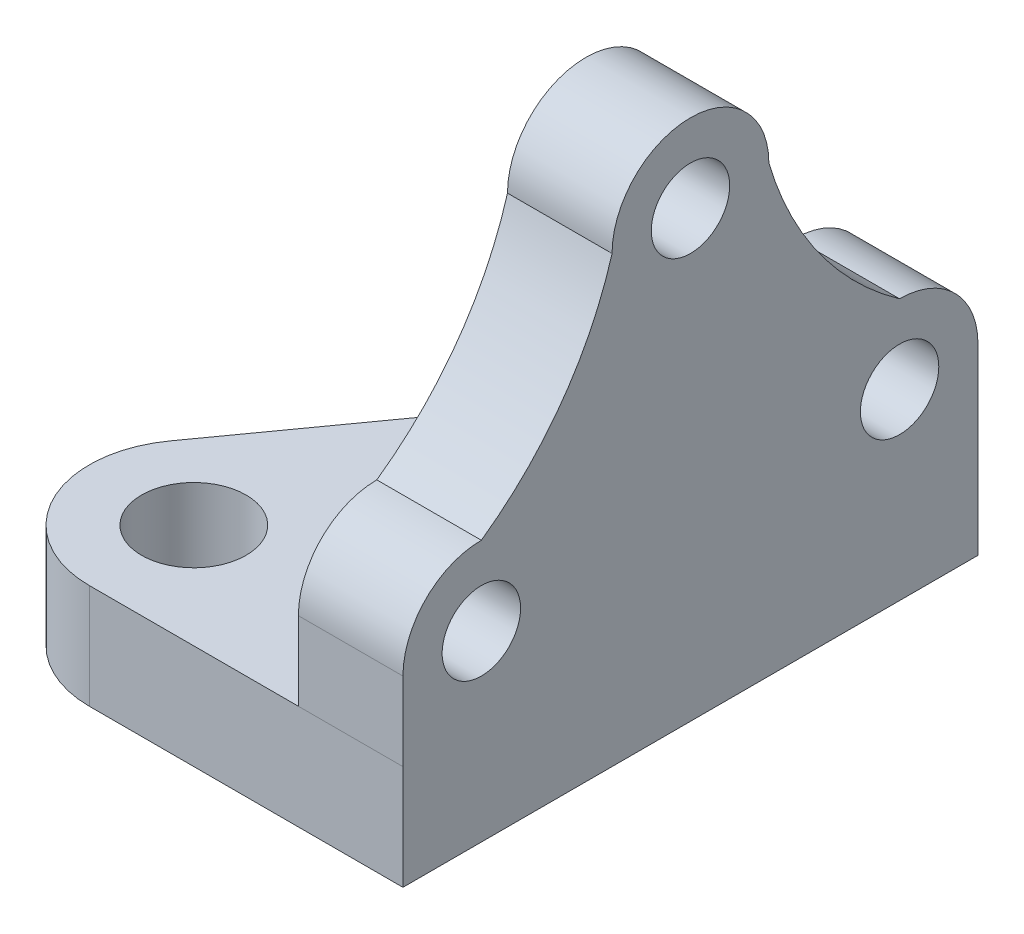
ISO-10303-21;
HEADER;
FILE_DESCRIPTION(('STEP AP214'),'2;1');
FILE_NAME('part.step','',(''),(''),'','','');
FILE_SCHEMA(('AUTOMOTIVE_DESIGN { 1 0 10303 214 1 1 1 1 }'));
ENDSEC;
DATA;
#1=APPLICATION_CONTEXT('core data for automotive mechanical design processes');
#2=APPLICATION_PROTOCOL_DEFINITION('international standard','automotive_design',2000,#1);
#3=PRODUCT_CONTEXT('',#1,'mechanical');
#4=PRODUCT('Part','Part','',(#3));
#5=PRODUCT_RELATED_PRODUCT_CATEGORY('part','',(#4));
#6=PRODUCT_DEFINITION_FORMATION('','',#4);
#7=PRODUCT_DEFINITION_CONTEXT('part definition',#1,'design');
#8=PRODUCT_DEFINITION('design','',#6,#7);
#9=PRODUCT_DEFINITION_SHAPE('','',#8);
#10=(LENGTH_UNIT() NAMED_UNIT(*) SI_UNIT(.MILLI.,.METRE.));
#11=(NAMED_UNIT(*) PLANE_ANGLE_UNIT() SI_UNIT($,.RADIAN.));
#12=(NAMED_UNIT(*) SI_UNIT($,.STERADIAN.) SOLID_ANGLE_UNIT());
#13=UNCERTAINTY_MEASURE_WITH_UNIT(LENGTH_MEASURE(1.E-05),#10,'distance_accuracy_value','');
#14=(GEOMETRIC_REPRESENTATION_CONTEXT(3) GLOBAL_UNCERTAINTY_ASSIGNED_CONTEXT((#13)) GLOBAL_UNIT_ASSIGNED_CONTEXT((#10,
#11,#12)) REPRESENTATION_CONTEXT('',''));
#15=CARTESIAN_POINT('',(0.,0.,0.));
#16=DIRECTION('',(0.,0.,1.));
#17=DIRECTION('',(1.,0.,0.));
#18=AXIS2_PLACEMENT_3D('',#15,#16,#17);
#19=CARTESIAN_POINT('',(20.,68.1526978623619,-77.4137770073067));
#20=DIRECTION('',(1.,0.,0.));
#21=DIRECTION('',(0.,0.,-1.));
#22=AXIS2_PLACEMENT_3D('',#19,#20,#21);
#23=PLANE('',#22);
#24=CARTESIAN_POINT('',(20.,0.,-40.));
#25=DIRECTION('',(1.,0.,0.));
#26=DIRECTION('',(0.,0.,-1.));
#27=AXIS2_PLACEMENT_3D('',#24,#25,#26);
#28=CIRCLE('',#27,7.5);
#29=CARTESIAN_POINT('',(20.,0.,-47.5));
#30=VERTEX_POINT('',#29);
#31=EDGE_CURVE('E154',#30,#30,#28,.T.);
#32=ORIENTED_EDGE('',*,*,#31,.F.);
#33=EDGE_LOOP('',(#32));
#34=FACE_BOUND('',#33,.T.);
#35=CARTESIAN_POINT('',(20.,68.1526978623619,-77.4137770073067));
#36=DIRECTION('',(-1.,0.,0.));
#37=DIRECTION('',(0.,0.,-1.));
#38=AXIS2_PLACEMENT_3D('',#35,#36,#37);
#39=CIRCLE('',#38,65.);
#40=CARTESIAN_POINT('',(20.,15.,-40.));
#41=VERTEX_POINT('',#40);
#42=CARTESIAN_POINT('',(20.,50.,-15.));
#43=VERTEX_POINT('',#42);
#44=EDGE_CURVE('E170',#41,#43,#39,.T.);
#45=ORIENTED_EDGE('',*,*,#44,.T.);
#46=CARTESIAN_POINT('',(20.,50.,0.));
#47=DIRECTION('',(1.,0.,0.));
#48=DIRECTION('',(0.,0.,-1.));
#49=AXIS2_PLACEMENT_3D('',#46,#47,#48);
#50=CIRCLE('',#49,15.);
#51=CARTESIAN_POINT('',(20.,50.,15.));
#52=VERTEX_POINT('',#51);
#53=EDGE_CURVE('E100',#43,#52,#50,.T.);
#54=ORIENTED_EDGE('',*,*,#53,.T.);
#55=CARTESIAN_POINT('',(20.,68.1526978623619,77.4137770073067));
#56=DIRECTION('',(-1.,0.,0.));
#57=DIRECTION('',(0.,0.,1.));
#58=AXIS2_PLACEMENT_3D('',#55,#56,#57);
#59=CIRCLE('',#58,65.);
#60=CARTESIAN_POINT('',(20.,15.,40.));
#61=VERTEX_POINT('',#60);
#62=EDGE_CURVE('E168',#52,#61,#59,.T.);
#63=ORIENTED_EDGE('',*,*,#62,.T.);
#64=CARTESIAN_POINT('',(20.,0.,40.));
#65=DIRECTION('',(1.,0.,0.));
#66=DIRECTION('',(0.,0.,-1.));
#67=AXIS2_PLACEMENT_3D('',#64,#65,#66);
#68=CIRCLE('',#67,15.);
#69=CARTESIAN_POINT('',(20.,0.,55.));
#70=VERTEX_POINT('',#69);
#71=EDGE_CURVE('E116',#61,#70,#68,.T.);
#72=ORIENTED_EDGE('',*,*,#71,.T.);
#73=DIRECTION('',(0.,-0.999999995009303,9.9906924504711E-05));
#74=VECTOR('',#73,1.);
#75=CARTESIAN_POINT('',(20.,-15.,55.001498603875));
#76=LINE('',#75,#74);
#77=CARTESIAN_POINT('',(20.,-15.,55.001498603875));
#78=VERTEX_POINT('',#77);
#79=EDGE_CURVE('E112',#70,#78,#76,.T.);
#80=ORIENTED_EDGE('',*,*,#79,.T.);
#81=DIRECTION('',(0.,1.,0.));
#82=VECTOR('',#81,1.);
#83=CARTESIAN_POINT('',(20.,-35.,55.001498603875));
#84=LINE('',#83,#82);
#85=CARTESIAN_POINT('',(20.,-35.,55.001498603875));
#86=VERTEX_POINT('',#85);
#87=EDGE_CURVE('E119',#86,#78,#84,.T.);
#88=ORIENTED_EDGE('',*,*,#87,.F.);
#89=DIRECTION('',(0.,0.,1.));
#90=VECTOR('',#89,1.);
#91=CARTESIAN_POINT('',(20.,-35.,-55.));
#92=LINE('',#91,#90);
#93=CARTESIAN_POINT('',(20.,-35.,-55.));
#94=VERTEX_POINT('',#93);
#95=EDGE_CURVE('E415',#94,#86,#92,.T.);
#96=ORIENTED_EDGE('',*,*,#95,.F.);
#97=DIRECTION('',(0.,1.,0.));
#98=VECTOR('',#97,1.);
#99=CARTESIAN_POINT('',(20.,0.,-55.));
#100=LINE('',#99,#98);
#101=CARTESIAN_POINT('',(20.,0.,-55.));
#102=VERTEX_POINT('',#101);
#103=EDGE_CURVE('E122',#94,#102,#100,.T.);
#104=ORIENTED_EDGE('',*,*,#103,.T.);
#105=CARTESIAN_POINT('',(20.,0.,-40.));
#106=DIRECTION('',(1.,0.,0.));
#107=DIRECTION('',(0.,0.,-1.));
#108=AXIS2_PLACEMENT_3D('',#105,#106,#107);
#109=CIRCLE('',#108,15.);
#110=EDGE_CURVE('E57',#102,#41,#109,.T.);
#111=ORIENTED_EDGE('',*,*,#110,.T.);
#112=EDGE_LOOP('',(#45,#54,#63,#72,#80,#88,#96,#104,#111));
#113=FACE_BOUND('',#112,.T.);
#114=CARTESIAN_POINT('',(20.,50.,0.));
#115=DIRECTION('',(1.,0.,0.));
#116=DIRECTION('',(0.,0.,-1.));
#117=AXIS2_PLACEMENT_3D('',#114,#115,#116);
#118=CIRCLE('',#117,7.5);
#119=CARTESIAN_POINT('',(20.,50.,-7.5));
#120=VERTEX_POINT('',#119);
#121=EDGE_CURVE('E161',#120,#120,#118,.T.);
#122=ORIENTED_EDGE('',*,*,#121,.F.);
#123=EDGE_LOOP('',(#122));
#124=FACE_BOUND('',#123,.T.);
#125=CARTESIAN_POINT('',(20.,0.,40.));
#126=DIRECTION('',(1.,0.,0.));
#127=DIRECTION('',(0.,0.,-1.));
#128=AXIS2_PLACEMENT_3D('',#125,#126,#127);
#129=CIRCLE('',#128,7.5);
#130=CARTESIAN_POINT('',(20.,0.,32.5));
#131=VERTEX_POINT('',#130);
#132=EDGE_CURVE('E144',#131,#131,#129,.T.);
#133=ORIENTED_EDGE('',*,*,#132,.F.);
#134=EDGE_LOOP('',(#133));
#135=FACE_BOUND('',#134,.T.);
#136=ADVANCED_FACE('F39',(#34,#113,#124,#135),#23,.T.);
#137=CARTESIAN_POINT('',(0.,68.1526978623619,-77.4137770073067));
#138=DIRECTION('',(1.,0.,0.));
#139=DIRECTION('',(0.,0.,-1.));
#140=AXIS2_PLACEMENT_3D('',#137,#138,#139);
#141=PLANE('',#140);
#142=CARTESIAN_POINT('',(0.,68.1526978623619,-77.4137770073067));
#143=DIRECTION('',(-1.,0.,0.));
#144=DIRECTION('',(0.,0.,-1.));
#145=AXIS2_PLACEMENT_3D('',#142,#143,#144);
#146=CIRCLE('',#145,65.);
#147=CARTESIAN_POINT('',(0.,15.,-40.));
#148=VERTEX_POINT('',#147);
#149=CARTESIAN_POINT('',(0.,50.,-15.));
#150=VERTEX_POINT('',#149);
#151=EDGE_CURVE('E163',#148,#150,#146,.T.);
#152=ORIENTED_EDGE('',*,*,#151,.F.);
#153=CARTESIAN_POINT('',(0.,0.,-40.));
#154=DIRECTION('',(1.,0.,0.));
#155=DIRECTION('',(0.,0.,-1.));
#156=AXIS2_PLACEMENT_3D('',#153,#154,#155);
#157=CIRCLE('',#156,15.);
#158=CARTESIAN_POINT('',(0.,0.,-55.));
#159=VERTEX_POINT('',#158);
#160=EDGE_CURVE('E90',#159,#148,#157,.T.);
#161=ORIENTED_EDGE('',*,*,#160,.F.);
#162=DIRECTION('',(0.,1.,0.));
#163=VECTOR('',#162,1.);
#164=CARTESIAN_POINT('',(0.,0.,-55.));
#165=LINE('',#164,#163);
#166=CARTESIAN_POINT('',(0.,-15.,-55.));
#167=VERTEX_POINT('',#166);
#168=EDGE_CURVE('E83',#167,#159,#165,.T.);
#169=ORIENTED_EDGE('',*,*,#168,.F.);
#170=DIRECTION('',(0.,0.,-1.));
#171=VECTOR('',#170,1.);
#172=CARTESIAN_POINT('',(0.,-15.,-55.));
#173=LINE('',#172,#171);
#174=CARTESIAN_POINT('',(0.,-15.,55.001498603875));
#175=VERTEX_POINT('',#174);
#176=EDGE_CURVE('E183',#175,#167,#173,.T.);
#177=ORIENTED_EDGE('',*,*,#176,.F.);
#178=DIRECTION('',(0.,-0.999999995009303,9.9906924504711E-05));
#179=VECTOR('',#178,1.);
#180=CARTESIAN_POINT('',(0.,-15.,55.001498603875));
#181=LINE('',#180,#179);
#182=CARTESIAN_POINT('',(0.,0.,55.));
#183=VERTEX_POINT('',#182);
#184=EDGE_CURVE('E128',#183,#175,#181,.T.);
#185=ORIENTED_EDGE('',*,*,#184,.F.);
#186=CARTESIAN_POINT('',(0.,0.,40.));
#187=DIRECTION('',(1.,0.,0.));
#188=DIRECTION('',(0.,0.,-1.));
#189=AXIS2_PLACEMENT_3D('',#186,#187,#188);
#190=CIRCLE('',#189,15.);
#191=CARTESIAN_POINT('',(0.,15.,40.));
#192=VERTEX_POINT('',#191);
#193=EDGE_CURVE('E185',#192,#183,#190,.T.);
#194=ORIENTED_EDGE('',*,*,#193,.F.);
#195=CARTESIAN_POINT('',(0.,68.1526978623619,77.4137770073067));
#196=DIRECTION('',(-1.,0.,0.));
#197=DIRECTION('',(0.,0.,1.));
#198=AXIS2_PLACEMENT_3D('',#195,#196,#197);
#199=CIRCLE('',#198,65.);
#200=CARTESIAN_POINT('',(0.,50.,15.));
#201=VERTEX_POINT('',#200);
#202=EDGE_CURVE('E179',#201,#192,#199,.T.);
#203=ORIENTED_EDGE('',*,*,#202,.F.);
#204=CARTESIAN_POINT('',(0.,50.,0.));
#205=DIRECTION('',(1.,0.,0.));
#206=DIRECTION('',(0.,0.,-1.));
#207=AXIS2_PLACEMENT_3D('',#204,#205,#206);
#208=CIRCLE('',#207,15.);
#209=EDGE_CURVE('E178',#150,#201,#208,.T.);
#210=ORIENTED_EDGE('',*,*,#209,.F.);
#211=EDGE_LOOP('',(#152,#161,#169,#177,#185,#194,#203,#210));
#212=FACE_BOUND('',#211,.T.);
#213=CARTESIAN_POINT('',(0.,50.,0.));
#214=DIRECTION('',(1.,0.,0.));
#215=DIRECTION('',(0.,0.,-1.));
#216=AXIS2_PLACEMENT_3D('',#213,#214,#215);
#217=CIRCLE('',#216,7.5);
#218=CARTESIAN_POINT('',(0.,50.,-7.5));
#219=VERTEX_POINT('',#218);
#220=EDGE_CURVE('E158',#219,#219,#217,.T.);
#221=ORIENTED_EDGE('',*,*,#220,.T.);
#222=EDGE_LOOP('',(#221));
#223=FACE_BOUND('',#222,.T.);
#224=CARTESIAN_POINT('',(0.,0.,-40.));
#225=DIRECTION('',(1.,0.,0.));
#226=DIRECTION('',(0.,0.,-1.));
#227=AXIS2_PLACEMENT_3D('',#224,#225,#226);
#228=CIRCLE('',#227,7.5);
#229=CARTESIAN_POINT('',(0.,0.,-47.5));
#230=VERTEX_POINT('',#229);
#231=EDGE_CURVE('E153',#230,#230,#228,.T.);
#232=ORIENTED_EDGE('',*,*,#231,.T.);
#233=EDGE_LOOP('',(#232));
#234=FACE_BOUND('',#233,.T.);
#235=CARTESIAN_POINT('',(0.,0.,40.));
#236=DIRECTION('',(1.,0.,0.));
#237=DIRECTION('',(0.,0.,-1.));
#238=AXIS2_PLACEMENT_3D('',#235,#236,#237);
#239=CIRCLE('',#238,7.5);
#240=CARTESIAN_POINT('',(0.,0.,32.5));
#241=VERTEX_POINT('',#240);
#242=EDGE_CURVE('E143',#241,#241,#239,.T.);
#243=ORIENTED_EDGE('',*,*,#242,.T.);
#244=EDGE_LOOP('',(#243));
#245=FACE_BOUND('',#244,.T.);
#246=ADVANCED_FACE('F204',(#212,#223,#234,#245),#141,.F.);
#247=CARTESIAN_POINT('',(20.,68.1526978623619,-77.4137770073067));
#248=DIRECTION('',(-1.,0.,0.));
#249=DIRECTION('',(0.,0.,1.));
#250=AXIS2_PLACEMENT_3D('',#247,#248,#249);
#251=CYLINDRICAL_SURFACE('',#250,65.);
#252=ORIENTED_EDGE('',*,*,#151,.T.);
#253=DIRECTION('',(-1.,0.,0.));
#254=VECTOR('',#253,1.);
#255=CARTESIAN_POINT('',(20.,50.,-15.));
#256=LINE('',#255,#254);
#257=EDGE_CURVE('E11',#43,#150,#256,.T.);
#258=ORIENTED_EDGE('',*,*,#257,.F.);
#259=ORIENTED_EDGE('',*,*,#44,.F.);
#260=DIRECTION('',(-1.,0.,0.));
#261=VECTOR('',#260,1.);
#262=CARTESIAN_POINT('',(20.,15.,-40.));
#263=LINE('',#262,#261);
#264=EDGE_CURVE('E171',#41,#148,#263,.T.);
#265=ORIENTED_EDGE('',*,*,#264,.T.);
#266=EDGE_LOOP('',(#252,#258,#259,#265));
#267=FACE_BOUND('',#266,.T.);
#268=ADVANCED_FACE('F41',(#267),#251,.F.);
#269=CARTESIAN_POINT('',(20.,50.,0.));
#270=DIRECTION('',(-1.,0.,0.));
#271=DIRECTION('',(0.,0.,1.));
#272=AXIS2_PLACEMENT_3D('',#269,#270,#271);
#273=CYLINDRICAL_SURFACE('',#272,15.);
#274=ORIENTED_EDGE('',*,*,#209,.T.);
#275=DIRECTION('',(-1.,0.,0.));
#276=VECTOR('',#275,1.);
#277=CARTESIAN_POINT('',(20.,50.,15.));
#278=LINE('',#277,#276);
#279=EDGE_CURVE('E48',#52,#201,#278,.T.);
#280=ORIENTED_EDGE('',*,*,#279,.F.);
#281=ORIENTED_EDGE('',*,*,#53,.F.);
#282=ORIENTED_EDGE('',*,*,#257,.T.);
#283=EDGE_LOOP('',(#274,#280,#281,#282));
#284=FACE_BOUND('',#283,.T.);
#285=ADVANCED_FACE('F220',(#284),#273,.T.);
#286=CARTESIAN_POINT('',(20.,68.1526978623619,77.4137770073067));
#287=DIRECTION('',(-1.,0.,0.));
#288=DIRECTION('',(0.,0.,1.));
#289=AXIS2_PLACEMENT_3D('',#286,#287,#288);
#290=CYLINDRICAL_SURFACE('',#289,65.);
#291=ORIENTED_EDGE('',*,*,#202,.T.);
#292=DIRECTION('',(-1.,0.,0.));
#293=VECTOR('',#292,1.);
#294=CARTESIAN_POINT('',(20.,15.,40.));
#295=LINE('',#294,#293);
#296=EDGE_CURVE('E193',#61,#192,#295,.T.);
#297=ORIENTED_EDGE('',*,*,#296,.F.);
#298=ORIENTED_EDGE('',*,*,#62,.F.);
#299=ORIENTED_EDGE('',*,*,#279,.T.);
#300=EDGE_LOOP('',(#291,#297,#298,#299));
#301=FACE_BOUND('',#300,.T.);
#302=ADVANCED_FACE('F200',(#301),#290,.F.);
#303=CARTESIAN_POINT('',(20.,0.,40.));
#304=DIRECTION('',(-1.,0.,0.));
#305=DIRECTION('',(0.,0.,1.));
#306=AXIS2_PLACEMENT_3D('',#303,#304,#305);
#307=CYLINDRICAL_SURFACE('',#306,15.);
#308=ORIENTED_EDGE('',*,*,#193,.T.);
#309=DIRECTION('',(-1.,0.,0.));
#310=VECTOR('',#309,1.);
#311=CARTESIAN_POINT('',(20.,0.,55.));
#312=LINE('',#311,#310);
#313=EDGE_CURVE('E135',#70,#183,#312,.T.);
#314=ORIENTED_EDGE('',*,*,#313,.F.);
#315=ORIENTED_EDGE('',*,*,#71,.F.);
#316=ORIENTED_EDGE('',*,*,#296,.T.);
#317=EDGE_LOOP('',(#308,#314,#315,#316));
#318=FACE_BOUND('',#317,.T.);
#319=ADVANCED_FACE('F210',(#318),#307,.T.);
#320=CARTESIAN_POINT('',(20.,-15.,55.001498603875));
#321=DIRECTION('',(0.,-9.9906924504711E-05,-0.999999995009303));
#322=DIRECTION('',(0.,0.999999995009303,-9.9906924504711E-05));
#323=AXIS2_PLACEMENT_3D('',#320,#321,#322);
#324=PLANE('',#323);
#325=ORIENTED_EDGE('',*,*,#184,.T.);
#326=DIRECTION('',(-1.,0.,0.));
#327=VECTOR('',#326,1.);
#328=CARTESIAN_POINT('',(20.,-15.,55.001498603875));
#329=LINE('',#328,#327);
#330=EDGE_CURVE('E130',#78,#175,#329,.T.);
#331=ORIENTED_EDGE('',*,*,#330,.F.);
#332=ORIENTED_EDGE('',*,*,#79,.F.);
#333=ORIENTED_EDGE('',*,*,#313,.T.);
#334=EDGE_LOOP('',(#325,#331,#332,#333));
#335=FACE_BOUND('',#334,.T.);
#336=ADVANCED_FACE('F126',(#335),#324,.F.);
#337=CARTESIAN_POINT('',(20.,0.,-55.));
#338=DIRECTION('',(0.,0.,1.));
#339=DIRECTION('',(1.,0.,0.));
#340=AXIS2_PLACEMENT_3D('',#337,#338,#339);
#341=PLANE('',#340);
#342=ORIENTED_EDGE('',*,*,#168,.T.);
#343=DIRECTION('',(-1.,0.,0.));
#344=VECTOR('',#343,1.);
#345=CARTESIAN_POINT('',(20.,0.,-55.));
#346=LINE('',#345,#344);
#347=EDGE_CURVE('E131',#102,#159,#346,.T.);
#348=ORIENTED_EDGE('',*,*,#347,.F.);
#349=ORIENTED_EDGE('',*,*,#103,.F.);
#350=DIRECTION('',(1.,0.,0.));
#351=VECTOR('',#350,1.);
#352=CARTESIAN_POINT('',(20.,-35.,-55.));
#353=LINE('',#352,#351);
#354=CARTESIAN_POINT('',(0.,-35.,-55.));
#355=VERTEX_POINT('',#354);
#356=EDGE_CURVE('E395',#355,#94,#353,.T.);
#357=ORIENTED_EDGE('',*,*,#356,.F.);
#358=DIRECTION('',(0.,1.,0.));
#359=VECTOR('',#358,1.);
#360=CARTESIAN_POINT('',(0.,-35.,-55.));
#361=LINE('',#360,#359);
#362=EDGE_CURVE('E393',#355,#167,#361,.T.);
#363=ORIENTED_EDGE('',*,*,#362,.T.);
#364=EDGE_LOOP('',(#342,#348,#349,#357,#363));
#365=FACE_BOUND('',#364,.T.);
#366=ADVANCED_FACE('F214',(#365),#341,.F.);
#367=CARTESIAN_POINT('',(20.,0.,-40.));
#368=DIRECTION('',(-1.,0.,0.));
#369=DIRECTION('',(0.,0.,1.));
#370=AXIS2_PLACEMENT_3D('',#367,#368,#369);
#371=CYLINDRICAL_SURFACE('',#370,15.);
#372=ORIENTED_EDGE('',*,*,#160,.T.);
#373=ORIENTED_EDGE('',*,*,#264,.F.);
#374=ORIENTED_EDGE('',*,*,#110,.F.);
#375=ORIENTED_EDGE('',*,*,#347,.T.);
#376=EDGE_LOOP('',(#372,#373,#374,#375));
#377=FACE_BOUND('',#376,.T.);
#378=ADVANCED_FACE('F235',(#377),#371,.T.);
#379=CARTESIAN_POINT('',(20.,50.,0.));
#380=DIRECTION('',(-1.,0.,0.));
#381=DIRECTION('',(0.,0.,1.));
#382=AXIS2_PLACEMENT_3D('',#379,#380,#381);
#383=CYLINDRICAL_SURFACE('',#382,7.5);
#384=ORIENTED_EDGE('',*,*,#121,.T.);
#385=EDGE_LOOP('',(#384));
#386=FACE_BOUND('',#385,.T.);
#387=ORIENTED_EDGE('',*,*,#220,.F.);
#388=EDGE_LOOP('',(#387));
#389=FACE_BOUND('',#388,.T.);
#390=ADVANCED_FACE('F230',(#386,#389),#383,.F.);
#391=CARTESIAN_POINT('',(20.,0.,-40.));
#392=DIRECTION('',(-1.,0.,0.));
#393=DIRECTION('',(0.,0.,1.));
#394=AXIS2_PLACEMENT_3D('',#391,#392,#393);
#395=CYLINDRICAL_SURFACE('',#394,7.5);
#396=ORIENTED_EDGE('',*,*,#31,.T.);
#397=EDGE_LOOP('',(#396));
#398=FACE_BOUND('',#397,.T.);
#399=ORIENTED_EDGE('',*,*,#231,.F.);
#400=EDGE_LOOP('',(#399));
#401=FACE_BOUND('',#400,.T.);
#402=ADVANCED_FACE('F306',(#398,#401),#395,.F.);
#403=CARTESIAN_POINT('',(20.,0.,40.));
#404=DIRECTION('',(-1.,0.,0.));
#405=DIRECTION('',(0.,0.,1.));
#406=AXIS2_PLACEMENT_3D('',#403,#404,#405);
#407=CYLINDRICAL_SURFACE('',#406,7.5);
#408=ORIENTED_EDGE('',*,*,#132,.T.);
#409=EDGE_LOOP('',(#408));
#410=FACE_BOUND('',#409,.T.);
#411=ORIENTED_EDGE('',*,*,#242,.F.);
#412=EDGE_LOOP('',(#411));
#413=FACE_BOUND('',#412,.T.);
#414=ADVANCED_FACE('F248',(#410,#413),#407,.F.);
#415=CARTESIAN_POINT('',(-40.,-15.,35.001498603875));
#416=DIRECTION('',(0.,-1.,0.));
#417=DIRECTION('',(0.,0.,-1.));
#418=AXIS2_PLACEMENT_3D('',#415,#416,#417);
#419=PLANE('',#418);
#420=CARTESIAN_POINT('',(-40.,-15.,35.001498603875));
#421=DIRECTION('',(0.,-1.,0.));
#422=DIRECTION('',(0.,0.,-1.));
#423=AXIS2_PLACEMENT_3D('',#420,#421,#422);
#424=CIRCLE('',#423,10.);
#425=CARTESIAN_POINT('',(-40.,-15.,25.001498603875));
#426=VERTEX_POINT('',#425);
#427=EDGE_CURVE('E418',#426,#426,#424,.T.);
#428=ORIENTED_EDGE('',*,*,#427,.T.);
#429=EDGE_LOOP('',(#428));
#430=FACE_BOUND('',#429,.T.);
#431=DIRECTION('',(-1.,0.,0.));
#432=VECTOR('',#431,1.);
#433=CARTESIAN_POINT('',(-40.,-15.,55.001498603875));
#434=LINE('',#433,#432);
#435=CARTESIAN_POINT('',(-40.,-15.,55.001498603875));
#436=VERTEX_POINT('',#435);
#437=EDGE_CURVE('E390',#175,#436,#434,.T.);
#438=ORIENTED_EDGE('',*,*,#437,.F.);
#439=ORIENTED_EDGE('',*,*,#176,.T.);
#440=DIRECTION('',(0.583235968180871,0.,-0.812302779399481));
#441=VECTOR('',#440,1.);
#442=CARTESIAN_POINT('',(0.,-15.,-55.));
#443=LINE('',#442,#441);
#444=CARTESIAN_POINT('',(-56.2460395562641,-15.,23.33675691208));
#445=VERTEX_POINT('',#444);
#446=EDGE_CURVE('E387',#445,#167,#443,.T.);
#447=ORIENTED_EDGE('',*,*,#446,.F.);
#448=CARTESIAN_POINT('',(-40.,-15.,35.001498603875));
#449=DIRECTION('',(0.,-1.,0.));
#450=DIRECTION('',(0.,0.,-1.));
#451=AXIS2_PLACEMENT_3D('',#448,#449,#450);
#452=CIRCLE('',#451,20.);
#453=EDGE_CURVE('E391',#436,#445,#452,.T.);
#454=ORIENTED_EDGE('',*,*,#453,.F.);
#455=EDGE_LOOP('',(#438,#439,#447,#454));
#456=FACE_BOUND('',#455,.T.);
#457=ADVANCED_FACE('F245',(#430,#456),#419,.F.);
#458=CARTESIAN_POINT('',(-40.,-35.,35.001498603875));
#459=DIRECTION('',(0.,-1.,0.));
#460=DIRECTION('',(0.,0.,-1.));
#461=AXIS2_PLACEMENT_3D('',#458,#459,#460);
#462=PLANE('',#461);
#463=ORIENTED_EDGE('',*,*,#356,.T.);
#464=ORIENTED_EDGE('',*,*,#95,.T.);
#465=DIRECTION('',(-1.,0.,0.));
#466=VECTOR('',#465,1.);
#467=CARTESIAN_POINT('',(20.,-35.,55.001498603875));
#468=LINE('',#467,#466);
#469=CARTESIAN_POINT('',(-40.,-35.,55.001498603875));
#470=VERTEX_POINT('',#469);
#471=EDGE_CURVE('E139',#86,#470,#468,.T.);
#472=ORIENTED_EDGE('',*,*,#471,.T.);
#473=CARTESIAN_POINT('',(-40.,-35.,35.001498603875));
#474=DIRECTION('',(0.,-1.,0.));
#475=DIRECTION('',(0.,0.,-1.));
#476=AXIS2_PLACEMENT_3D('',#473,#474,#475);
#477=CIRCLE('',#476,20.);
#478=CARTESIAN_POINT('',(-56.2460395562641,-35.,23.33675691208));
#479=VERTEX_POINT('',#478);
#480=EDGE_CURVE('E405',#470,#479,#477,.T.);
#481=ORIENTED_EDGE('',*,*,#480,.T.);
#482=DIRECTION('',(0.583235968180871,0.,-0.812302779399481));
#483=VECTOR('',#482,1.);
#484=CARTESIAN_POINT('',(0.,-35.,-55.));
#485=LINE('',#484,#483);
#486=EDGE_CURVE('E397',#479,#355,#485,.T.);
#487=ORIENTED_EDGE('',*,*,#486,.T.);
#488=EDGE_LOOP('',(#463,#464,#472,#481,#487));
#489=FACE_BOUND('',#488,.T.);
#490=CARTESIAN_POINT('',(-40.,-35.,35.001498603875));
#491=DIRECTION('',(0.,-1.,0.));
#492=DIRECTION('',(0.,0.,-1.));
#493=AXIS2_PLACEMENT_3D('',#490,#491,#492);
#494=CIRCLE('',#493,10.);
#495=CARTESIAN_POINT('',(-40.,-35.,25.001498603875));
#496=VERTEX_POINT('',#495);
#497=EDGE_CURVE('E409',#496,#496,#494,.T.);
#498=ORIENTED_EDGE('',*,*,#497,.F.);
#499=EDGE_LOOP('',(#498));
#500=FACE_BOUND('',#499,.T.);
#501=ADVANCED_FACE('F250',(#489,#500),#462,.T.);
#502=CARTESIAN_POINT('',(-40.,-35.,55.001498603875));
#503=DIRECTION('',(0.,0.,-1.));
#504=DIRECTION('',(-1.,0.,0.));
#505=AXIS2_PLACEMENT_3D('',#502,#503,#504);
#506=PLANE('',#505);
#507=ORIENTED_EDGE('',*,*,#330,.T.);
#508=ORIENTED_EDGE('',*,*,#437,.T.);
#509=DIRECTION('',(0.,1.,0.));
#510=VECTOR('',#509,1.);
#511=CARTESIAN_POINT('',(-40.,-35.,55.001498603875));
#512=LINE('',#511,#510);
#513=EDGE_CURVE('E142',#470,#436,#512,.T.);
#514=ORIENTED_EDGE('',*,*,#513,.F.);
#515=ORIENTED_EDGE('',*,*,#471,.F.);
#516=ORIENTED_EDGE('',*,*,#87,.T.);
#517=EDGE_LOOP('',(#507,#508,#514,#515,#516));
#518=FACE_BOUND('',#517,.T.);
#519=ADVANCED_FACE('F140',(#518),#506,.F.);
#520=CARTESIAN_POINT('',(-40.,-35.,35.001498603875));
#521=DIRECTION('',(0.,1.,0.));
#522=DIRECTION('',(0.,0.,1.));
#523=AXIS2_PLACEMENT_3D('',#520,#521,#522);
#524=CYLINDRICAL_SURFACE('',#523,20.);
#525=ORIENTED_EDGE('',*,*,#453,.T.);
#526=DIRECTION('',(0.,1.,0.));
#527=VECTOR('',#526,1.);
#528=CARTESIAN_POINT('',(-56.2460395562641,-35.,23.33675691208));
#529=LINE('',#528,#527);
#530=EDGE_CURVE('E146',#479,#445,#529,.T.);
#531=ORIENTED_EDGE('',*,*,#530,.F.);
#532=ORIENTED_EDGE('',*,*,#480,.F.);
#533=ORIENTED_EDGE('',*,*,#513,.T.);
#534=EDGE_LOOP('',(#525,#531,#532,#533));
#535=FACE_BOUND('',#534,.T.);
#536=ADVANCED_FACE('F266',(#535),#524,.T.);
#537=CARTESIAN_POINT('',(0.,-35.,-55.));
#538=DIRECTION('',(0.812302779399481,0.,0.583235968180871));
#539=DIRECTION('',(0.583235968180871,0.,-0.812302779399481));
#540=AXIS2_PLACEMENT_3D('',#537,#538,#539);
#541=PLANE('',#540);
#542=ORIENTED_EDGE('',*,*,#446,.T.);
#543=ORIENTED_EDGE('',*,*,#362,.F.);
#544=ORIENTED_EDGE('',*,*,#486,.F.);
#545=ORIENTED_EDGE('',*,*,#530,.T.);
#546=EDGE_LOOP('',(#542,#543,#544,#545));
#547=FACE_BOUND('',#546,.T.);
#548=ADVANCED_FACE('F272',(#547),#541,.F.);
#549=CARTESIAN_POINT('',(-40.,-35.,35.001498603875));
#550=DIRECTION('',(0.,1.,0.));
#551=DIRECTION('',(0.,0.,1.));
#552=AXIS2_PLACEMENT_3D('',#549,#550,#551);
#553=CYLINDRICAL_SURFACE('',#552,10.);
#554=ORIENTED_EDGE('',*,*,#497,.T.);
#555=EDGE_LOOP('',(#554));
#556=FACE_BOUND('',#555,.T.);
#557=ORIENTED_EDGE('',*,*,#427,.F.);
#558=EDGE_LOOP('',(#557));
#559=FACE_BOUND('',#558,.T.);
#560=ADVANCED_FACE('F284',(#556,#559),#553,.F.);
#561=CLOSED_SHELL('',(#136,#246,#268,#285,#302,#319,#336,#366,#378,#390,#402,#414,#457,#501,
#519,#536,#548,#560));
#562=MANIFOLD_SOLID_BREP('B2',#561);
#563=ADVANCED_BREP_SHAPE_REPRESENTATION('',(#18,#562),#14);
#564=SHAPE_DEFINITION_REPRESENTATION(#9,#563);
ENDSEC;
END-ISO-10303-21;
